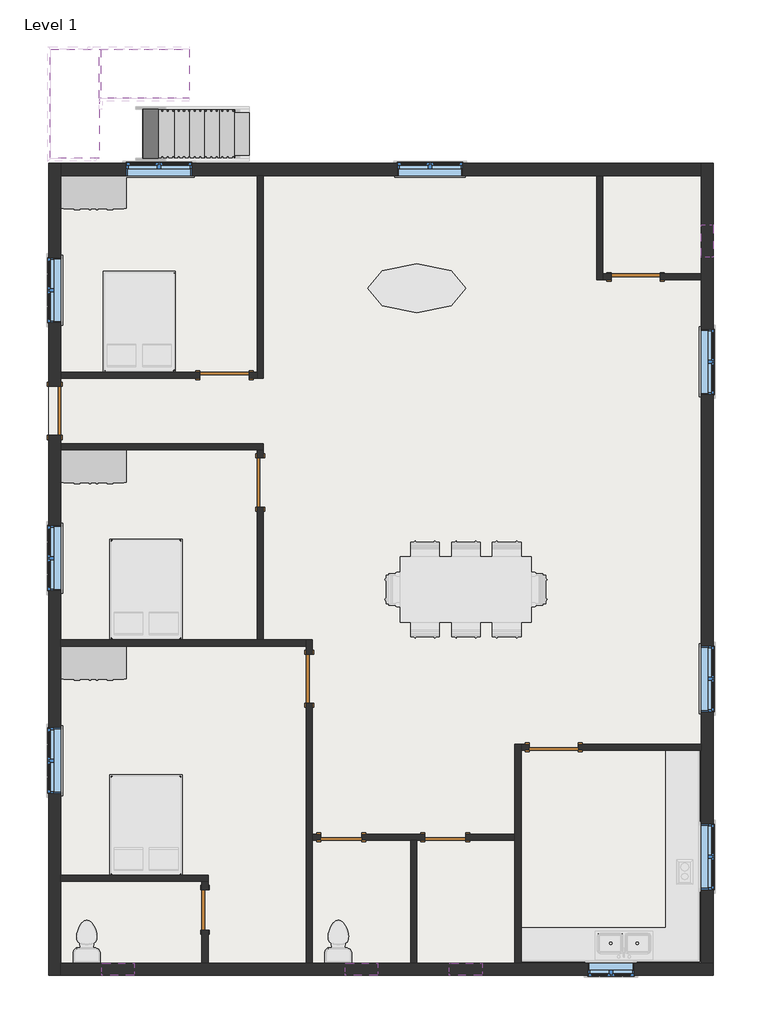
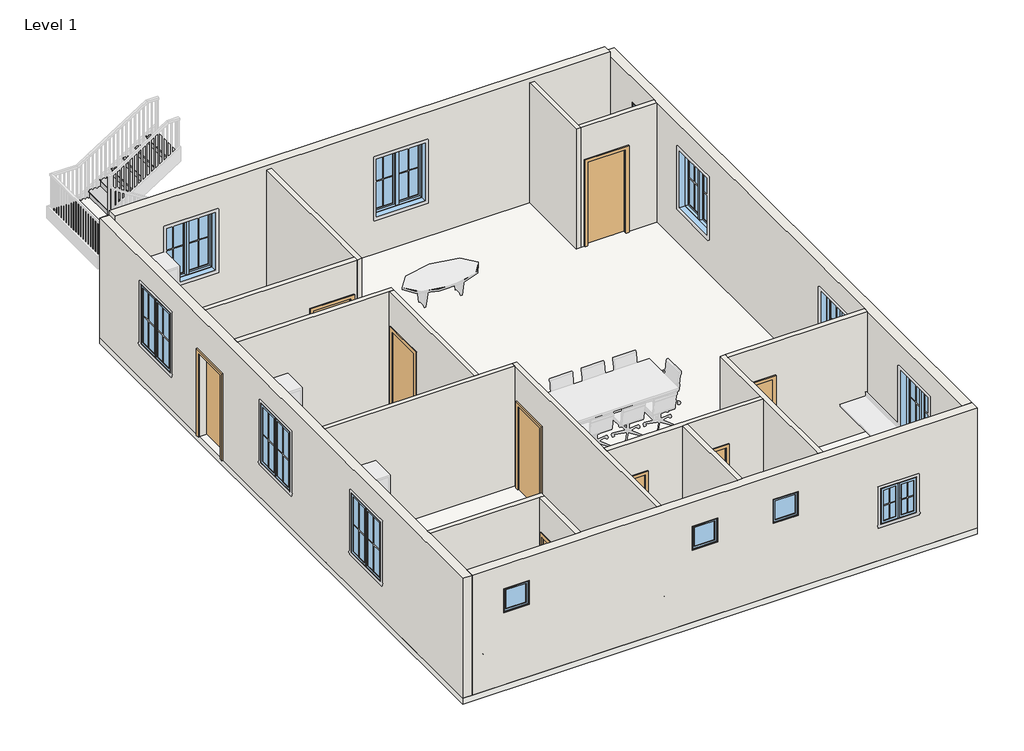
# One storey, part 1 of 3: 18 walls, 13 windows, 9 doors, 2 slabs, 2 stair flights.
"""IFC4 building model written with IfcOpenShell, lengths in millimetres."""

from ifc_helpers import new_model, si_unit, frame, origin, origin_with_axes, place, context, project, spatial, polyline, outline, extrude, faceted_brep, transform, mapped, element, save
from components import door_214872d5, door_a90ba1ad, door_e5f9f3c4, door_305aa2a5, non_monolithic_landing_2ab6d15e, stair_flight_b5a9fedd, stair_flight_7eff537e, window_80340324, window_339605e1, window_8377141f

model = new_model("IFC4")

# Units and contexts
model_context = context("Model", 3, world=origin())
ifc_project = project(units=[si_unit("LENGTHUNIT", "METRE", prefix="MILLI")], contexts=[model_context])

# Site, building, storey
site = spatial("IfcSite", under=ifc_project)
building = spatial("IfcBuilding", under=site)
storey = spatial("IfcBuildingStorey", under=building, Name="Level 1", Elevation=0.0)

# Doors
placement = place(None, origin())
door_shape = door_214872d5(model_context)
element("IfcDoor", 1, ObjectType="Single-Flush : 30\" x 84\"", at=placement, inside=storey, context=model_context, shape_type="MappedRepresentation", body=[
    mapped(door_shape, transform((15054.6713581, 8240.8164065, 0.0), x_axis=(-1.0, 0.0, 0.0), y_axis=(0.0, -1.0, 0.0), z_axis=(0.0, 0.0, 1.0))),
])
element("IfcDoor", 2, ObjectType="Single-Flush : 30\" x 84\"", at=placement, inside=storey, context=model_context, shape_type="MappedRepresentation", body=[
    mapped(door_shape, transform((16997.7713581, 8240.8164065, 0.0), x_axis=(-1.0, 0.0, 0.0), y_axis=(0.0, -1.0, 0.0), z_axis=(0.0, 0.0, 1.0))),
])
element("IfcDoor", 3, ObjectType="Single-Flush : 30\" x 84\"", at=placement, inside=storey, context=model_context, shape_type="MappedRepresentation", body=[
    mapped(door_shape, transform((12521.0213581, 6888.2664065, 0.0), x_axis=(0.0, 1.0, 0.0), y_axis=(-1.0, 0.0, 0.0), z_axis=(0.0, 0.0, 1.0))),
])
door_2_shape = door_a90ba1ad(model_context)
element("IfcDoor", 4, ObjectType="Single-Flush : 36\" x 84\"", at=placement, inside=storey, context=model_context, shape_type="MappedRepresentation", body=[
    mapped(door_2_shape, transform((9720.6713581, 16184.6664065, 0.0), x_axis=(0.0, 1.0, 0.0), y_axis=(-1.0, 0.0, 0.0), z_axis=(0.0, 0.0, 1.0))),
])
door_3_shape = door_e5f9f3c4(model_context)
element("IfcDoor", 5, ObjectType="Single-Flush : 36\" x 84\"", at=placement, inside=storey, context=model_context, shape_type="MappedRepresentation", body=[
    mapped(door_3_shape, transform((12882.9713581, 16851.4164065, 0.0), x_axis=(1.0, 0.0, 0.0), y_axis=(0.0, 1.0, 0.0), z_axis=(0.0, 0.0, 1.0))),
])
element("IfcDoor", 6, ObjectType="Single-Flush : 36\" x 84\"", at=placement, inside=storey, context=model_context, shape_type="MappedRepresentation", body=[
    mapped(door_3_shape, transform((13549.7213581, 14851.1664065, 0.0), x_axis=(0.0, 1.0, 0.0), y_axis=(-1.0, 0.0, 0.0), z_axis=(0.0, 0.0, 1.0))),
])
element("IfcDoor", 7, ObjectType="Single-Flush : 36\" x 84\"", at=placement, inside=storey, context=model_context, shape_type="MappedRepresentation", body=[
    mapped(door_3_shape, transform((14464.1213581, 11193.5664065, 0.0), x_axis=(0.0, 1.0, 0.0), y_axis=(-1.0, 0.0, 0.0), z_axis=(0.0, 0.0, 1.0))),
])
element("IfcDoor", 8, ObjectType="Single-Flush : 36\" x 84\"", at=placement, inside=storey, context=model_context, shape_type="MappedRepresentation", body=[
    mapped(door_3_shape, transform((19017.0713581, 9917.2164065, 0.0), x_axis=(-1.0, 0.0, 0.0), y_axis=(0.0, -1.0, 0.0), z_axis=(0.0, 0.0, 1.0))),
])
door_4_shape = door_305aa2a5(model_context)
element("IfcDoor", 9, ObjectType="Single-Flush : 36\" x 84\"", at=placement, inside=storey, context=model_context, shape_type="MappedRepresentation", body=[
    mapped(door_4_shape, transform((20541.0713581, 18680.2164065, 0.0), x_axis=(-1.0, 0.0, 0.0), y_axis=(0.0, -1.0, 0.0), z_axis=(0.0, 0.0, 1.0))),
])

# Slabs
element("IfcSlab", 10, at=placement, inside=storey, context=model_context, shape_type="SweptSolid", body=[
    extrude(outline(polyline([(21988.8713581, 20794.7664065), (21988.8713581, 5669.0664065), (9606.3713581, 5669.0664065), (9606.3713581, 20794.7664065), (21988.8713581, 20794.7664065)])), frame((0.0, 0.0, -152.4), z_axis=(0.0, 0.0, 1.0), x_axis=(1.0, 0.0, 0.0)), (0.0, 0.0, 1.0), 152.4),
])
non_monolithic_landing_shape = non_monolithic_landing_2ab6d15e(model_context)
element("IfcSlab", 11, ObjectType="Non-Monolithic Landing", at=placement, inside=storey, context=model_context, shape_type="MappedRepresentation", body=[
    mapped(non_monolithic_landing_shape, transform((0.0, 0.0, 0.0), x_axis=(1.0, 0.0, 0.0), y_axis=(0.0, 1.0, 0.0), z_axis=(0.0, 0.0, 1.0))),
])

# Stair flights
stair_flight_shape = stair_flight_b5a9fedd(model_context)
element("IfcStairFlight", 12, ObjectType="2\" Tread 1\" Nosing 1/4\" Riser", at=placement, inside=storey, context=model_context, shape_type="MappedRepresentation", body=[
    mapped(stair_flight_shape, transform((0.0, 0.0, 0.0), x_axis=(1.0, 0.0, 0.0), y_axis=(0.0, 1.0, 0.0), z_axis=(0.0, 0.0, 1.0))),
])
stair_flight_2_shape = stair_flight_7eff537e(model_context)
element("IfcStairFlight", 13, ObjectType="2\" Tread 1\" Nosing 1/4\" Riser", at=placement, inside=storey, context=model_context, shape_type="MappedRepresentation", body=[
    mapped(stair_flight_2_shape, transform((0.0, 0.0, 0.0), x_axis=(1.0, 0.0, 0.0), y_axis=(0.0, 1.0, 0.0), z_axis=(0.0, 0.0, 1.0))),
])

# Walls
element("IfcWall", 14, at=placement, inside=storey, context=model_context, shape_type="Brep", body=[
    faceted_brep([(9606.3713581, 20794.7664065, 0.0), (9606.3713581, 16641.8664065, 0.0), (9606.3713581, 16641.8664065, 2133.6), (9606.3713581, 15727.4664065, 2133.6), (9606.3713581, 15727.4664065, 0.0), (9606.3713581, 5669.0664065, 0.0), (9606.3713581, 5669.0664065, 3048.0), (9606.3713581, 20788.4164065, 3048.0), (9606.3713581, 20794.7664065, 3048.0), (9606.3713581, 19042.1664065, 2438.4), (9606.3713581, 17822.9664065, 2438.4), (9606.3713581, 17822.9664065, 914.4), (9606.3713581, 19042.1664065, 914.4), (9606.3713581, 14051.0664065, 2438.4), (9606.3713581, 12831.8664065, 2438.4), (9606.3713581, 12831.8664065, 914.4), (9606.3713581, 14051.0664065, 914.4), (9606.3713581, 10279.1664065, 2438.4), (9606.3713581, 9059.9664065, 2438.4), (9606.3713581, 9059.9664065, 914.4), (9606.3713581, 10279.1664065, 914.4), (9834.9713581, 16641.8664065, 2133.6), (9834.9713581, 16641.8664065, 0.0), (9834.9713581, 16794.2664065, 0.0), (9834.9713581, 16908.5664065, 0.0), (9834.9713581, 20566.1664065, 0.0), (9834.9713581, 20794.7664065, 0.0), (9834.9713581, 20794.7664065, 3048.0), (9834.9713581, 20788.4164065, 3048.0), (9834.9713581, 16908.5664065, 3048.0), (9834.9713581, 16794.2664065, 3048.0), (9834.9713581, 15575.0664065, 3048.0), (9834.9713581, 15460.7664065, 3048.0), (9834.9713581, 11917.4664065, 3048.0), (9834.9713581, 11803.1664065, 3048.0), (9834.9713581, 7535.9664065, 3048.0), (9834.9713581, 7421.6664065, 3048.0), (9834.9713581, 5897.6664065, 3048.0), (9834.9713581, 5669.0664065, 3048.0), (9834.9713581, 5669.0664065, 0.0), (9834.9713581, 5897.6664065, 0.0), (9834.9713581, 7421.6664065, 0.0), (9834.9713581, 7535.9664065, 0.0), (9834.9713581, 11803.1664065, 0.0), (9834.9713581, 11917.4664065, 0.0), (9834.9713581, 15460.7664065, 0.0), (9834.9713581, 15575.0664065, 0.0), (9834.9713581, 15727.4664065, 0.0), (9834.9713581, 15727.4664065, 2133.6), (9834.9713581, 19042.1664065, 2438.4), (9834.9713581, 19042.1664065, 914.4), (9834.9713581, 17822.9664065, 914.4), (9834.9713581, 17822.9664065, 2438.4), (9834.9713581, 14051.0664065, 2438.4), (9834.9713581, 14051.0664065, 914.4), (9834.9713581, 12831.8664065, 914.4), (9834.9713581, 12831.8664065, 2438.4), (9834.9713581, 10279.1664065, 2438.4), (9834.9713581, 10279.1664065, 914.4), (9834.9713581, 9059.9664065, 914.4), (9834.9713581, 9059.9664065, 2438.4)], [[[0, 1, 2, 3, 4, 5, 6, 7, 8], [9, 10, 11, 12], [13, 14, 15, 16], [17, 18, 19, 20]], [[21, 22, 23, 24, 25, 26, 27, 28, 29, 30, 31, 32, 33, 34, 35, 36, 37, 38, 39, 40, 41, 42, 43, 44, 45, 46, 47, 48], [49, 50, 51, 52], [53, 54, 55, 56], [57, 58, 59, 60]], [[26, 25, 24, 23, 22, 1, 0]], [[47, 46, 45, 44, 43, 42, 41, 40, 39, 5, 4]], [[0, 8, 27, 26]], [[6, 5, 39, 38]], [[2, 1, 22, 21]], [[3, 2, 21, 48]], [[4, 3, 48, 47]], [[50, 49, 9, 12]], [[51, 50, 12, 11]], [[52, 51, 11, 10]], [[49, 52, 10, 9]], [[54, 53, 13, 16]], [[55, 54, 16, 15]], [[56, 55, 15, 14]], [[53, 56, 14, 13]], [[58, 57, 17, 20]], [[59, 58, 20, 19]], [[60, 59, 19, 18]], [[57, 60, 18, 17]], [[8, 7, 28, 27]], [[7, 6, 38, 37, 36, 35, 34, 33, 32, 31, 30, 29, 28]]]),
])
element("IfcWall", 15, at=placement, inside=storey, context=model_context, shape_type="Brep", body=[
    faceted_brep([(9834.9713581, 20566.1664065, 0.0), (13492.5713581, 20566.1664065, 0.0), (13606.8713581, 20566.1664065, 0.0), (19817.1713581, 20566.1664065, 0.0), (19931.4713581, 20566.1664065, 0.0), (21760.2713581, 20566.1664065, 0.0), (21760.2713581, 20566.1664065, 3155.7444843), (9834.9713581, 20566.1664065, 3155.7444843), (12273.3713581, 20566.1664065, 2438.4), (12273.3713581, 20566.1664065, 914.4), (11054.1713581, 20566.1664065, 914.4), (11054.1713581, 20566.1664065, 2438.4), (17321.6213581, 20566.1664065, 2438.4), (17321.6213581, 20566.1664065, 914.4), (16102.4213581, 20566.1664065, 914.4), (16102.4213581, 20566.1664065, 2438.4), (9834.9713581, 20794.7664065, 0.0), (9834.9713581, 20794.7664065, 3048.0), (9834.9713581, 20794.7664065, 3155.7444843), (21760.2713581, 20794.7664065, 3155.7444843), (21760.2713581, 20794.7664065, 3048.0), (21760.2713581, 20794.7664065, 0.0), (12273.3713581, 20794.7664065, 2438.4), (11054.1713581, 20794.7664065, 2438.4), (11054.1713581, 20794.7664065, 914.4), (12273.3713581, 20794.7664065, 914.4), (17321.6213581, 20794.7664065, 2438.4), (16102.4213581, 20794.7664065, 2438.4), (16102.4213581, 20794.7664065, 914.4), (17321.6213581, 20794.7664065, 914.4)], [[[0, 1, 2, 3, 4, 5, 6, 7], [8, 9, 10, 11], [12, 13, 14, 15]], [[16, 17, 18, 19, 20, 21], [22, 23, 24, 25], [26, 27, 28, 29]], [[5, 4, 3, 2, 1, 0, 16, 21]], [[7, 6, 19, 18]], [[0, 7, 18, 17, 16]], [[6, 5, 21, 20, 19]], [[9, 8, 22, 25]], [[10, 9, 25, 24]], [[11, 10, 24, 23]], [[8, 11, 23, 22]], [[13, 12, 26, 29]], [[14, 13, 29, 28]], [[15, 14, 28, 27]], [[12, 15, 27, 26]]]),
])
element("IfcWall", 16, at=placement, inside=storey, context=model_context, shape_type="Brep", body=[
    faceted_brep([(13492.5713581, 20566.1664065, 0.0), (13492.5713581, 16908.5664065, 0.0), (13492.5713581, 16794.2664065, 0.0), (13492.5713581, 16794.2664065, 3048.0), (13492.5713581, 16908.5664065, 3048.0), (13492.5713581, 20566.1664065, 3048.0), (13606.8713581, 20566.1664065, 0.0), (13606.8713581, 20566.1664065, 3048.0), (13606.8713581, 16794.2664065, 3048.0), (13606.8713581, 16794.2664065, 0.0)], [[[0, 1, 2, 3, 4, 5]], [[6, 7, 8, 9]], [[2, 1, 0, 6, 9]], [[3, 2, 9, 8]], [[0, 5, 7, 6]], [[5, 4, 3, 8, 7]]]),
])
element("IfcWall", 17, at=placement, inside=storey, context=model_context, shape_type="SweptSolid", body=[
    extrude(outline(polyline([(2133.6, 13340.1713581), (0.0, 13340.1713581), (0.0, 13492.5713581), (3048.0, 13492.5713581), (3048.0, 9834.9713581), (0.0, 9834.9713581), (0.0, 12425.7713581), (2133.6, 12425.7713581), (2133.6, 13340.1713581)])), frame((0.0, 16794.2664065, 0.0), z_axis=(0.0, 1.0, 0.0), x_axis=(0.0, 0.0, 1.0)), (0.0, 0.0, 1.0), 114.3),
])
element("IfcWall", 18, at=placement, inside=storey, context=model_context, shape_type="Brep", body=[
    faceted_brep([(9834.9713581, 15460.7664065, 0.0), (13492.5713581, 15460.7664065, 0.0), (13606.8713581, 15460.7664065, 0.0), (13606.8713581, 15460.7664065, 3048.0), (13492.5713581, 15460.7664065, 3048.0), (9834.9713581, 15460.7664065, 3048.0), (9834.9713581, 15575.0664065, 0.0), (9834.9713581, 15575.0664065, 3048.0), (13606.8713581, 15575.0664065, 3048.0), (13606.8713581, 15575.0664065, 0.0)], [[[0, 1, 2, 3, 4, 5]], [[6, 7, 8, 9]], [[2, 1, 0, 6, 9]], [[0, 5, 7, 6]], [[3, 2, 9, 8]], [[5, 4, 3, 8, 7]]]),
])
element("IfcWall", 19, at=placement, inside=storey, context=model_context, shape_type="Brep", body=[
    faceted_brep([(9834.9713581, 11803.1664065, 0.0), (14406.9713581, 11803.1664065, 0.0), (14406.9713581, 11803.1664065, 3048.0), (9834.9713581, 11803.1664065, 3048.0), (9834.9713581, 11917.4664065, 0.0), (9834.9713581, 11917.4664065, 3048.0), (13492.5713581, 11917.4664065, 3048.0), (13606.8713581, 11917.4664065, 3048.0), (14406.9713581, 11917.4664065, 3048.0), (14406.9713581, 11917.4664065, 0.0), (13606.8713581, 11917.4664065, 0.0), (13492.5713581, 11917.4664065, 0.0)], [[[0, 1, 2, 3]], [[4, 5, 6, 7, 8, 9, 10, 11]], [[1, 0, 4, 11, 10, 9]], [[0, 3, 5, 4]], [[2, 1, 9, 8]], [[3, 2, 8, 7, 6, 5]]]),
])
element("IfcWall", 20, at=placement, inside=storey, context=model_context, shape_type="SweptSolid", body=[
    extrude(outline(polyline([(15460.7664065, 0.0), (15308.3664065, 0.0), (15308.3664065, 2133.6), (14393.9664065, 2133.6), (14393.9664065, 0.0), (11917.4664065, 0.0), (11917.4664065, 3048.0), (15460.7664065, 3048.0), (15460.7664065, 0.0)])), frame((13492.5713581, 0.0, 0.0), z_axis=(1.0, 0.0, 0.0), x_axis=(0.0, 1.0, 0.0)), (0.0, 0.0, 1.0), 114.3),
])
element("IfcWall", 21, at=placement, inside=storey, context=model_context, shape_type="Brep", body=[
    faceted_brep([(9834.9713581, 7421.6664065, 0.0), (12463.8713581, 7421.6664065, 0.0), (12578.1713581, 7421.6664065, 0.0), (12578.1713581, 7421.6664065, 3048.0), (12463.8713581, 7421.6664065, 3048.0), (9834.9713581, 7421.6664065, 3048.0), (9834.9713581, 7535.9664065, 0.0), (9834.9713581, 7535.9664065, 3048.0), (12578.1713581, 7535.9664065, 3048.0), (12578.1713581, 7535.9664065, 0.0)], [[[0, 1, 2, 3, 4, 5]], [[6, 7, 8, 9]], [[2, 1, 0, 6, 9]], [[0, 5, 7, 6]], [[5, 4, 3, 8, 7]], [[3, 2, 9, 8]]]),
])
element("IfcWall", 22, at=placement, inside=storey, context=model_context, shape_type="Brep", body=[
    faceted_brep([(14521.2713581, 11650.7664065, 2133.6), (14521.2713581, 11650.7664065, 0.0), (14521.2713581, 11917.4664065, 0.0), (14521.2713581, 11917.4664065, 3048.0), (14521.2713581, 8297.9664065, 3048.0), (14521.2713581, 8183.6664065, 3048.0), (14521.2713581, 5897.6664065, 3048.0), (14521.2713581, 5897.6664065, 0.0), (14521.2713581, 8183.6664065, 0.0), (14521.2713581, 8297.9664065, 0.0), (14521.2713581, 10736.3664065, 0.0), (14521.2713581, 10736.3664065, 2133.6), (14406.9713581, 11917.4664065, 0.0), (14406.9713581, 11803.1664065, 0.0), (14406.9713581, 11650.7664065, 0.0), (14406.9713581, 11650.7664065, 2133.6), (14406.9713581, 10736.3664065, 2133.6), (14406.9713581, 10736.3664065, 0.0), (14406.9713581, 5897.6664065, 0.0), (14406.9713581, 5897.6664065, 3048.0), (14406.9713581, 11803.1664065, 3048.0), (14406.9713581, 11917.4664065, 3048.0)], [[[0, 1, 2, 3, 4, 5, 6, 7, 8, 9, 10, 11]], [[12, 13, 14, 15, 16, 17, 18, 19, 20, 21]], [[2, 1, 14, 13, 12]], [[10, 9, 8, 7, 18, 17]], [[3, 2, 12, 21]], [[7, 6, 19, 18]], [[15, 14, 1, 0]], [[16, 15, 0, 11]], [[17, 16, 11, 10]], [[6, 5, 4, 3, 21, 20, 19]]]),
])
element("IfcWall", 23, at=placement, inside=storey, context=model_context, shape_type="Brep", body=[
    faceted_brep([(9834.9713581, 5669.0664065, 0.0), (21988.8713581, 5669.0664065, 0.0), (21988.8713581, 5669.0664065, 3048.0), (9834.9713581, 5669.0664065, 3048.0), (10596.9713581, 5669.0664065, 2438.4), (11206.5713581, 5669.0664065, 2438.4), (11206.5713581, 5669.0664065, 1828.8), (10596.9713581, 5669.0664065, 1828.8), (15130.8713581, 5669.0664065, 2438.4), (15740.4713581, 5669.0664065, 2438.4), (15740.4713581, 5669.0664065, 1828.8), (15130.8713581, 5669.0664065, 1828.8), (17073.9713581, 5669.0664065, 2438.4), (17683.5713581, 5669.0664065, 2438.4), (17683.5713581, 5669.0664065, 1828.8), (17073.9713581, 5669.0664065, 1828.8), (19652.0713581, 5669.0664065, 1828.8), (20515.6713581, 5669.0664065, 1828.8), (20515.6713581, 5669.0664065, 914.4), (19652.0713581, 5669.0664065, 914.4), (9834.9713581, 5897.6664065, 0.0), (9834.9713581, 5897.6664065, 3048.0), (12463.8713581, 5897.6664065, 3048.0), (12578.1713581, 5897.6664065, 3048.0), (14406.9713581, 5897.6664065, 3048.0), (14521.2713581, 5897.6664065, 3048.0), (16350.0713581, 5897.6664065, 3048.0), (16464.3713581, 5897.6664065, 3048.0), (18293.1713581, 5897.6664065, 3048.0), (18407.4713581, 5897.6664065, 3048.0), (21760.2713581, 5897.6664065, 3048.0), (21988.8713581, 5897.6664065, 3048.0), (21988.8713581, 5897.6664065, 0.0), (21760.2713581, 5897.6664065, 0.0), (18407.4713581, 5897.6664065, 0.0), (18293.1713581, 5897.6664065, 0.0), (16464.3713581, 5897.6664065, 0.0), (16350.0713581, 5897.6664065, 0.0), (14521.2713581, 5897.6664065, 0.0), (14406.9713581, 5897.6664065, 0.0), (12578.1713581, 5897.6664065, 0.0), (12463.8713581, 5897.6664065, 0.0), (10596.9713581, 5897.6664065, 2438.4), (10596.9713581, 5897.6664065, 1828.8), (11206.5713581, 5897.6664065, 1828.8), (11206.5713581, 5897.6664065, 2438.4), (15130.8713581, 5897.6664065, 2438.4), (15130.8713581, 5897.6664065, 1828.8), (15740.4713581, 5897.6664065, 1828.8), (15740.4713581, 5897.6664065, 2438.4), (17073.9713581, 5897.6664065, 2438.4), (17073.9713581, 5897.6664065, 1828.8), (17683.5713581, 5897.6664065, 1828.8), (17683.5713581, 5897.6664065, 2438.4), (19652.0713581, 5897.6664065, 1828.8), (19652.0713581, 5897.6664065, 914.4), (20515.6713581, 5897.6664065, 914.4), (20515.6713581, 5897.6664065, 1828.8)], [[[0, 1, 2, 3], [4, 5, 6, 7], [8, 9, 10, 11], [12, 13, 14, 15], [16, 17, 18, 19]], [[20, 21, 22, 23, 24, 25, 26, 27, 28, 29, 30, 31, 32, 33, 34, 35, 36, 37, 38, 39, 40, 41], [42, 43, 44, 45], [46, 47, 48, 49], [50, 51, 52, 53], [54, 55, 56, 57]], [[1, 0, 20, 41, 40, 39, 38, 37, 36, 35, 34, 33, 32]], [[0, 3, 21, 20]], [[2, 1, 32, 31]], [[43, 42, 4, 7]], [[44, 43, 7, 6]], [[45, 44, 6, 5]], [[42, 45, 5, 4]], [[47, 46, 8, 11]], [[48, 47, 11, 10]], [[49, 48, 10, 9]], [[46, 49, 9, 8]], [[51, 50, 12, 15]], [[52, 51, 15, 14]], [[53, 52, 14, 13]], [[50, 53, 13, 12]], [[55, 54, 16, 19]], [[56, 55, 19, 18]], [[57, 56, 18, 17]], [[54, 57, 17, 16]], [[3, 2, 31, 30, 29, 28, 27, 26, 25, 24, 23, 22, 21]]]),
])
element("IfcWall", 24, at=placement, inside=storey, context=model_context, shape_type="SweptSolid", body=[
    extrude(outline(polyline([(16464.3713581, 8183.6664065), (16464.3713581, 5897.6664065), (16350.0713581, 5897.6664065), (16350.0713581, 8183.6664065), (16464.3713581, 8183.6664065)])), origin_with_axes(), (0.0, 0.0, 1.0), 3048.0),
])
element("IfcWall", 25, at=placement, inside=storey, context=model_context, shape_type="Brep", body=[
    faceted_brep([(16616.7713581, 8297.9664065, 2133.6), (16616.7713581, 8297.9664065, 0.0), (15435.6713581, 8297.9664065, 0.0), (15435.6713581, 8297.9664065, 2133.6), (14673.6713581, 8297.9664065, 2133.6), (14673.6713581, 8297.9664065, 0.0), (14521.2713581, 8297.9664065, 0.0), (14521.2713581, 8297.9664065, 3048.0), (18293.1713581, 8297.9664065, 3048.0), (18293.1713581, 8297.9664065, 0.0), (17378.7713581, 8297.9664065, 0.0), (17378.7713581, 8297.9664065, 2133.6), (15435.6713581, 8183.6664065, 0.0), (16350.0713581, 8183.6664065, 0.0), (16464.3713581, 8183.6664065, 0.0), (16616.7713581, 8183.6664065, 0.0), (16616.7713581, 8183.6664065, 2133.6), (17378.7713581, 8183.6664065, 2133.6), (17378.7713581, 8183.6664065, 0.0), (18293.1713581, 8183.6664065, 0.0), (18293.1713581, 8183.6664065, 3048.0), (16464.3713581, 8183.6664065, 3048.0), (16350.0713581, 8183.6664065, 3048.0), (14521.2713581, 8183.6664065, 3048.0), (14521.2713581, 8183.6664065, 0.0), (14673.6713581, 8183.6664065, 0.0), (14673.6713581, 8183.6664065, 2133.6), (15435.6713581, 8183.6664065, 2133.6)], [[[0, 1, 2, 3, 4, 5, 6, 7, 8, 9, 10, 11]], [[12, 13, 14, 15, 16, 17, 18, 19, 20, 21, 22, 23, 24, 25, 26, 27]], [[6, 5, 25, 24]], [[10, 9, 19, 18]], [[2, 1, 15, 14, 13, 12]], [[7, 6, 24, 23]], [[9, 8, 20, 19]], [[26, 25, 5, 4]], [[27, 26, 4, 3]], [[12, 27, 3, 2]], [[16, 15, 1, 0]], [[17, 16, 0, 11]], [[18, 17, 11, 10]], [[8, 7, 23, 22, 21, 20]]]),
])
element("IfcWall", 26, at=placement, inside=storey, context=model_context, shape_type="Brep", body=[
    faceted_brep([(18293.1713581, 9974.3664065, 0.0), (18293.1713581, 8297.9664065, 0.0), (18293.1713581, 8183.6664065, 0.0), (18293.1713581, 5897.6664065, 0.0), (18293.1713581, 5897.6664065, 3048.0), (18293.1713581, 8183.6664065, 3048.0), (18293.1713581, 8297.9664065, 3048.0), (18293.1713581, 9974.3664065, 3048.0), (18407.4713581, 9974.3664065, 0.0), (18407.4713581, 9974.3664065, 3048.0), (18407.4713581, 9860.0664065, 3048.0), (18407.4713581, 5897.6664065, 3048.0), (18407.4713581, 5897.6664065, 0.0), (18407.4713581, 9860.0664065, 0.0)], [[[0, 1, 2, 3, 4, 5, 6, 7]], [[8, 9, 10, 11, 12, 13]], [[3, 2, 1, 0, 8, 13, 12]], [[4, 3, 12, 11]], [[0, 7, 9, 8]], [[7, 6, 5, 4, 11, 10, 9]]]),
])
element("IfcWall", 27, at=placement, inside=storey, context=model_context, shape_type="Brep", body=[
    faceted_brep([(21988.8713581, 5897.6664065, 0.0), (21988.8713581, 20794.7664065, 0.0), (21988.8713581, 20794.7664065, 3048.0), (21988.8713581, 5897.6664065, 3048.0), (21988.8713581, 10583.9664065, 2438.4), (21988.8713581, 11803.1664065, 2438.4), (21988.8713581, 11803.1664065, 914.4), (21988.8713581, 10583.9664065, 914.4), (21988.8713581, 16489.4664065, 2438.4), (21988.8713581, 17708.6664065, 2438.4), (21988.8713581, 17708.6664065, 914.4), (21988.8713581, 16489.4664065, 914.4), (21988.8713581, 19042.1664065, 2438.4), (21988.8713581, 19651.7664065, 2438.4), (21988.8713581, 19651.7664065, 1828.8), (21988.8713581, 19042.1664065, 1828.8), (21988.8713581, 7269.2664065, 2438.4), (21988.8713581, 8488.4664065, 2438.4), (21988.8713581, 8488.4664065, 914.4), (21988.8713581, 7269.2664065, 914.4), (21760.2713581, 5897.6664065, 0.0), (21760.2713581, 5897.6664065, 3048.0), (21760.2713581, 9860.0664065, 3048.0), (21760.2713581, 9974.3664065, 3048.0), (21760.2713581, 18623.0664065, 3048.0), (21760.2713581, 18737.3664065, 3048.0), (21760.2713581, 20794.7664065, 3048.0), (21760.2713581, 20794.7664065, 0.0), (21760.2713581, 20566.1664065, 0.0), (21760.2713581, 18737.3664065, 0.0), (21760.2713581, 18623.0664065, 0.0), (21760.2713581, 9974.3664065, 0.0), (21760.2713581, 9860.0664065, 0.0), (21760.2713581, 10583.9664065, 2438.4), (21760.2713581, 10583.9664065, 914.4), (21760.2713581, 11803.1664065, 914.4), (21760.2713581, 11803.1664065, 2438.4), (21760.2713581, 16489.4664065, 2438.4), (21760.2713581, 16489.4664065, 914.4), (21760.2713581, 17708.6664065, 914.4), (21760.2713581, 17708.6664065, 2438.4), (21760.2713581, 19042.1664065, 2438.4), (21760.2713581, 19042.1664065, 1828.8), (21760.2713581, 19651.7664065, 1828.8), (21760.2713581, 19651.7664065, 2438.4), (21760.2713581, 7269.2664065, 2438.4), (21760.2713581, 7269.2664065, 914.4), (21760.2713581, 8488.4664065, 914.4), (21760.2713581, 8488.4664065, 2438.4)], [[[0, 1, 2, 3], [4, 5, 6, 7], [8, 9, 10, 11], [12, 13, 14, 15], [16, 17, 18, 19]], [[20, 21, 22, 23, 24, 25, 26, 27, 28, 29, 30, 31, 32], [33, 34, 35, 36], [37, 38, 39, 40], [41, 42, 43, 44], [45, 46, 47, 48]], [[1, 0, 20, 32, 31, 30, 29, 28, 27]], [[0, 3, 21, 20]], [[2, 1, 27, 26]], [[34, 33, 4, 7]], [[35, 34, 7, 6]], [[36, 35, 6, 5]], [[33, 36, 5, 4]], [[38, 37, 8, 11]], [[39, 38, 11, 10]], [[40, 39, 10, 9]], [[37, 40, 9, 8]], [[42, 41, 12, 15]], [[43, 42, 15, 14]], [[44, 43, 14, 13]], [[41, 44, 13, 12]], [[46, 45, 16, 19]], [[47, 46, 19, 18]], [[48, 47, 18, 17]], [[45, 48, 17, 16]], [[3, 2, 26, 25, 24, 23, 22, 21]]]),
])
element("IfcWall", 28, at=placement, inside=storey, context=model_context, shape_type="SweptSolid", body=[
    extrude(outline(polyline([(0.0, 18407.4713581), (0.0, 18559.8713581), (2133.6, 18559.8713581), (2133.6, 19474.2713581), (0.0, 19474.2713581), (0.0, 21760.2713581), (3048.0, 21760.2713581), (3048.0, 18407.4713581), (0.0, 18407.4713581)])), frame((0.0, 9860.0664065, 0.0), z_axis=(0.0, 1.0, 0.0), x_axis=(0.0, 0.0, 1.0)), (0.0, 0.0, 1.0), 114.3),
])
element("IfcWall", 29, at=placement, inside=storey, context=model_context, shape_type="Brep", body=[
    faceted_brep([(19817.1713581, 20566.1664065, 0.0), (19817.1713581, 18623.0664065, 0.0), (19817.1713581, 18623.0664065, 3048.0), (19817.1713581, 20566.1664065, 3048.0), (19931.4713581, 20566.1664065, 0.0), (19931.4713581, 20566.1664065, 3048.0), (19931.4713581, 18737.3664065, 3048.0), (19931.4713581, 18623.0664065, 3048.0), (19931.4713581, 18623.0664065, 0.0), (19931.4713581, 18737.3664065, 0.0)], [[[0, 1, 2, 3]], [[4, 5, 6, 7, 8, 9]], [[1, 0, 4, 9, 8]], [[0, 3, 5, 4]], [[2, 1, 8, 7]], [[3, 2, 7, 6, 5]]]),
])
element("IfcWall", 30, at=placement, inside=storey, context=model_context, shape_type="SweptSolid", body=[
    extrude(outline(polyline([(0.0, 19931.4713581), (0.0, 20083.8713581), (2133.6, 20083.8713581), (2133.6, 20998.2713581), (0.0, 20998.2713581), (0.0, 21760.2713581), (3048.0, 21760.2713581), (3048.0, 19931.4713581), (0.0, 19931.4713581)])), frame((0.0, 18623.0664065, 0.0), z_axis=(0.0, 1.0, 0.0), x_axis=(0.0, 0.0, 1.0)), (0.0, 0.0, 1.0), 114.3),
])
element("IfcWall", 31, at=placement, inside=storey, context=model_context, shape_type="SweptSolid", body=[
    extrude(outline(polyline([(5897.6664065, 0.0), (5897.6664065, 3048.0), (7421.6664065, 3048.0), (7421.6664065, 0.0), (7269.2664065, 0.0), (7269.2664065, 2133.6), (6507.2664065, 2133.6), (6507.2664065, 0.0), (5897.6664065, 0.0)])), frame((12463.8713581, 0.0, 0.0), z_axis=(1.0, 0.0, 0.0), x_axis=(0.0, 1.0, 0.0)), (0.0, 0.0, 1.0), 114.3),
])

# Windows
window_shape = window_80340324(model_context)
element("IfcWindow", 32, ObjectType="Fixed : 24\" x 24\"", at=placement, inside=storey, context=model_context, shape_type="MappedRepresentation", body=[
    mapped(window_shape, transform((10863.6713581, 5783.3664065, 914.4), x_axis=(-1.0, 0.0, 0.0), y_axis=(0.0, -1.0, 0.0), z_axis=(0.0, 0.0, 1.0))),
])
element("IfcWindow", 33, ObjectType="Fixed : 24\" x 24\"", at=placement, inside=storey, context=model_context, shape_type="MappedRepresentation", body=[
    mapped(window_shape, transform((15397.5713581, 5783.3664065, 914.4), x_axis=(-1.0, 0.0, 0.0), y_axis=(0.0, -1.0, 0.0), z_axis=(0.0, 0.0, 1.0))),
])
element("IfcWindow", 34, ObjectType="Fixed : 24\" x 24\"", at=placement, inside=storey, context=model_context, shape_type="MappedRepresentation", body=[
    mapped(window_shape, transform((17340.6713581, 5783.3664065, 914.4), x_axis=(-1.0, 0.0, 0.0), y_axis=(0.0, -1.0, 0.0), z_axis=(0.0, 0.0, 1.0))),
])
element("IfcWindow", 35, ObjectType="Fixed : 24\" x 24\"", at=placement, inside=storey, context=model_context, shape_type="MappedRepresentation", body=[
    mapped(window_shape, transform((21874.5713581, 19308.8664065, 914.4), x_axis=(0.0, -1.0, 0.0), y_axis=(1.0, 0.0, 0.0), z_axis=(0.0, 0.0, 1.0))),
])
window_2_shape = window_339605e1(model_context)
element("IfcWindow", 36, ObjectType="Window-Casement-Double : 34\" x 36\"", at=placement, inside=storey, context=model_context, shape_type="MappedRepresentation", body=[
    mapped(window_2_shape, transform((20083.8713581, 5783.3664065, 0.0), x_axis=(-1.0, 0.0, 0.0), y_axis=(0.0, -1.0, 0.0), z_axis=(0.0, 0.0, 1.0))),
])
window_3_shape = window_8377141f(model_context)
element("IfcWindow", 37, ObjectType="Window-Casement-Double : 48\" x 60\"", at=placement, inside=storey, context=model_context, shape_type="MappedRepresentation", body=[
    mapped(window_3_shape, transform((9720.6713581, 18432.5664065, 0.0), x_axis=(0.0, 1.0, 0.0), y_axis=(-1.0, 0.0, 0.0), z_axis=(0.0, 0.0, 1.0))),
])
element("IfcWindow", 38, ObjectType="Window-Casement-Double : 48\" x 60\"", at=placement, inside=storey, context=model_context, shape_type="MappedRepresentation", body=[
    mapped(window_3_shape, transform((11663.7713581, 20680.4664065, 0.0), x_axis=(1.0, 0.0, 0.0), y_axis=(0.0, 1.0, 0.0), z_axis=(0.0, 0.0, 1.0))),
])
element("IfcWindow", 39, ObjectType="Window-Casement-Double : 48\" x 60\"", at=placement, inside=storey, context=model_context, shape_type="MappedRepresentation", body=[
    mapped(window_3_shape, transform((9720.6713581, 13441.4664065, 0.0), x_axis=(0.0, 1.0, 0.0), y_axis=(-1.0, 0.0, 0.0), z_axis=(0.0, 0.0, 1.0))),
])
element("IfcWindow", 40, ObjectType="Window-Casement-Double : 48\" x 60\"", at=placement, inside=storey, context=model_context, shape_type="MappedRepresentation", body=[
    mapped(window_3_shape, transform((9720.6713581, 9669.5664065, 0.0), x_axis=(0.0, 1.0, 0.0), y_axis=(-1.0, 0.0, 0.0), z_axis=(0.0, 0.0, 1.0))),
])
element("IfcWindow", 41, ObjectType="Window-Casement-Double : 48\" x 60\"", at=placement, inside=storey, context=model_context, shape_type="MappedRepresentation", body=[
    mapped(window_3_shape, transform((21874.5713581, 11193.5664065, 0.0), x_axis=(0.0, -1.0, 0.0), y_axis=(1.0, 0.0, 0.0), z_axis=(0.0, 0.0, 1.0))),
])
element("IfcWindow", 42, ObjectType="Window-Casement-Double : 48\" x 60\"", at=placement, inside=storey, context=model_context, shape_type="MappedRepresentation", body=[
    mapped(window_3_shape, transform((21874.5713581, 17099.0664065, 0.0), x_axis=(0.0, -1.0, 0.0), y_axis=(1.0, 0.0, 0.0), z_axis=(0.0, 0.0, 1.0))),
])
element("IfcWindow", 43, ObjectType="Window-Casement-Double : 48\" x 60\"", at=placement, inside=storey, context=model_context, shape_type="MappedRepresentation", body=[
    mapped(window_3_shape, transform((16712.0213581, 20680.4664065, 0.0), x_axis=(1.0, 0.0, 0.0), y_axis=(0.0, 1.0, 0.0), z_axis=(0.0, 0.0, 1.0))),
])
element("IfcWindow", 44, ObjectType="Window-Casement-Double : 48\" x 60\"", at=placement, inside=storey, context=model_context, shape_type="MappedRepresentation", body=[
    mapped(window_3_shape, transform((21874.5713581, 7878.8664065, 0.0), x_axis=(0.0, -1.0, 0.0), y_axis=(1.0, 0.0, 0.0), z_axis=(0.0, 0.0, 1.0))),
])

save(model, "model.ifc")

# Revit data of these elements
# Type "Single-Flush : 30\" x 84\""
#   Type Mark = "4"
#   Construction Type Id = "MDOOR"
#   Assembly Code = "C1020"
#   Analytic Construction = "Metal"
#   Thickness = 0' - 2"
#   Heat Transfer Coefficient (U) = 0.651978 BTU/(h·ft²·°F)
#   Height = 7' - 0"
#   Trim Projection Ext = 0' - 1"
#   Trim Projection Int = 0' - 1"
#   Trim Width = 0' - 3"
#   Width = 2' - 6"
#   Define Thermal Properties by = 1
#   Define Thermal Properties by = 1
#   Door Material = Door - Panel
#   Frame Material = Door - Frame
#   Visual Light Transmittance = 0
#   Solar Heat Gain Coefficient = 0
#   Function = (empty or 0)
#   Wall Closure = (empty or 0)
# Type "Single-Flush : 36\" x 84\""
#   Type Mark = "1"
#   Construction Type Id = "MDOOR"
#   Assembly Code = "C1020"
#   Analytic Construction = "Metal"
#   Thickness = 0' - 2"
#   Heat Transfer Coefficient (U) = 0.651978 BTU/(h·ft²·°F)
#   Height = 7' - 0"
#   Trim Projection Ext = 0' - 1"
#   Trim Projection Int = 0' - 1"
#   Trim Width = 0' - 3"
#   Width = 3' - 0"
#   Define Thermal Properties by = 1
#   Define Thermal Properties by = 1
#   Door Material = Door - Panel
#   Frame Material = Door - Frame
#   Visual Light Transmittance = 0
#   Solar Heat Gain Coefficient = 0
#   Function = (empty or 0)
#   Wall Closure = (empty or 0)
# Type
#   Assembly Code = "B1010"
#   Function = 0
#   Layers, outside or top first: 0' - 6" "Concrete, Cast-in-Place gray" (function 1)
# Type
#   Assembly Code = "B2010"
#   Layers, outside or top first: 0' - 9" no material (function 1)
# Type
#   Assembly Code = "B2010"
#   Layers, outside or top first: 0' - 4 1/2" no material (function 1)
# Type "Fixed : 24\" x 24\""
#   Type Mark = "3"
#   Construction Type Id = "GSP4R"
#   Assembly Code = "B2020100"
#   Analytic Construction = "1/8 in Pilkington single glazing"
#   Visual Light Transmittance = 0.9
#   Solar Heat Gain Coefficient = 0.78
#   Heat Transfer Coefficient (U) = 0.6496 BTU/(h·ft²·°F)
#   Height = 2' - 0"
#   Default Sill Height = 3' - 0"
#   Width = 2' - 0"
#   Window Inset = 0' - 0 3/4"
#   Define Thermal Properties by = 1
#   Define Thermal Properties by = 1
#   Glass Pane Material = Glass
#   Sash Material = Sash
#   Wall Closure = (empty or 0)
# Type "Window-Casement-Double : 34\" x 36\""
#   Type Mark = "14"
#   Fire Rating = "0.5h"
#   Assembly Code = "B2020100"
#   Analytic Construction = "Double glazing - domestic"
#   Frame Extension [instance default] = 0' - 0 1/4"
#   Window Inset [instance default] = 0' - 0"
#   Wall Thickness [instance default] = 0' - 6"
#   Interior Wall Closure [instance default] = 0' - 2 1/4"
#   Half Width = 1' - 5"
#   Visual Light Transmittance = 0.81
#   Thermal Resistance (R) = 1.8146 (h·ft²·°F)/BTU
#   Solar Heat Gain Coefficient = 0.76
#   Rough Width = 2' - 10 1/2"
#   Rough Height = 3' - 0 1/2"
#   Height = 3' - 0"
#   Heat Transfer Coefficient (U) = 0.5511 BTU/(h·ft²·°F)
#   Exterior Wall Closure [instance default] = 0' - 1 1/4"
#   Extension Jamb [instance default] = 0' - 2 1/4"
#   Default Sill Height = 3' - 0"
#   Width = 2' - 10"
#   Define Thermal Properties by = 0
#   Muntin Visibility = yes
#   Interior Trim Visibility [instance default] = yes
#   Exterior Trim Visibility [instance default] = yes
#   Extension Jamb Visibility [instance default] = yes
#   Interior Trim Material = Wood - Stained
#   Muntin Pattern = Muntin Pattern_2x2 : Muntin Pattern_2x2
#   Interior Trim = Trim-Window-Interior-Flat : Picture Frame
#   Interior Frame Material = Wood - Stained
#   Glass Panel Material = Glass
#   Exterior Trim Material = Clad - White
#   Exterior Trim = Trim-Window-Exterior-Flat : with Sill
#   Exterior Frame Material = Clad - White
#   Wall Closure = (empty or 0)
# Type "Window-Casement-Double : 48\" x 60\""
#   Type Mark = "16"
#   Fire Rating = "0.5h"
#   Assembly Code = "B2020100"
#   Analytic Construction = "Double glazing - domestic"
#   Frame Extension [instance default] = 0' - 0 1/4"
#   Window Inset [instance default] = 0' - 0"
#   Wall Thickness [instance default] = 0' - 6"
#   Interior Wall Closure [instance default] = 0' - 2 1/4"
#   Half Width = 2' - 0"
#   Visual Light Transmittance = 0.81
#   Thermal Resistance (R) = 1.8146 (h·ft²·°F)/BTU
#   Solar Heat Gain Coefficient = 0.76
#   Rough Width = 4' - 0 1/2"
#   Rough Height = 5' - 0 1/2"
#   Height = 5' - 0"
#   Heat Transfer Coefficient (U) = 0.5511 BTU/(h·ft²·°F)
#   Exterior Wall Closure [instance default] = 0' - 1 1/4"
#   Extension Jamb [instance default] = 0' - 2 1/4"
#   Default Sill Height = 3' - 0"
#   Width = 4' - 0"
#   Define Thermal Properties by = 0
#   Muntin Visibility = yes
#   Interior Trim Visibility [instance default] = yes
#   Exterior Trim Visibility [instance default] = yes
#   Extension Jamb Visibility [instance default] = yes
#   Interior Trim Material = Wood - Stained
#   Muntin Pattern = Muntin Pattern_2x2 : Muntin Pattern_2x2
#   Interior Trim = Trim-Window-Interior-Flat : Picture Frame
#   Interior Frame Material = Wood - Stained
#   Glass Panel Material = Glass
#   Exterior Trim Material = Clad - White
#   Exterior Trim = Trim-Window-Exterior-Flat : with Sill
#   Exterior Frame Material = Clad - White
#   Wall Closure = (empty or 0)
# Elements 1, 2, 3 (IfcDoor, "Single-Flush : 30\" x 84\"")
#   Phase Created = New Construction
#   Materials on its faces: "Door - Frame", "Door - Panel"
# Elements 4, 5, 6, 7, 8, 9 (IfcDoor, "Single-Flush : 36\" x 84\"")
#   Phase Created = New Construction
#   Materials on its faces: "Door - Frame", "Door - Panel"
# Element 10 (IfcSlab)
#   Height Offset From Level = 0' - 0"
#   Phase Created = New Construction
#   Materials on its faces: "Concrete, Cast-in-Place gray"
# Element 11 (IfcSlab, "Non-Monolithic Landing")
#   Phase Created = New Construction
# Elements 12, 13 (IfcStairFlight, "2\" Tread 1\" Nosing 1/4\" Riser")
#   Phase Created = New Construction
# Elements 14, 16, 17, 18, 19, 20, 21, 22, 23, 24, 25, 26, 27, 28, 29, 30, 31 (IfcWall)
#   Top Offset = 0' - 0"
#   Base Offset = 0' - 0"
#   wall height = 10' - 0"
#   Phase Created = New Construction
#   Base Constraint = Level 1
#   Top Constraint = Level 2
#   Materials on its faces: "Default Wall"
# Element 15 (IfcWall)
#   Top Offset = -0' - 1.75809"
#   Base Offset = 0' - 0"
#   wall height = 10' - 4.24191"
#   Phase Created = New Construction
#   Base Constraint = Level 1
#   Top Constraint = Level 2
#   Materials on its faces: "Default Wall"
# Element 32 (IfcWindow, "Fixed : 24\" x 24\"")
#   Mark = "5"
#   Phase Created = New Construction
#   Materials on its faces: "Sash", "Glass"
# Element 33 (IfcWindow, "Fixed : 24\" x 24\"")
#   Mark = "6"
#   Phase Created = New Construction
#   Materials on its faces: "Sash", "Glass"
# Element 34 (IfcWindow, "Fixed : 24\" x 24\"")
#   Mark = "7"
#   Phase Created = New Construction
#   Materials on its faces: "Sash", "Glass"
# Element 35 (IfcWindow, "Fixed : 24\" x 24\"")
#   Mark = "12"
#   Phase Created = New Construction
#   Materials on its faces: "Sash", "Glass"
# Element 36 (IfcWindow, "Window-Casement-Double : 34\" x 36\"")
#   Mark = "8"
#   Window Inset = 0' - 0"
#   Interior Wall Closure = 0' - 2 1/4"
#   Frame Extension = 0' - 0 1/4"
#   Exterior Wall Closure = 0' - 1 1/4"
#   Interior Trim Visibility = yes
#   Exterior Trim Visibility = yes
#   Phase Created = New Construction
#   Materials on its faces: "Wood - Stained", "Glass", "Clad - White"
# Element 37 (IfcWindow, "Window-Casement-Double : 48\" x 60\"")
#   Mark = "1"
#   Window Inset = 0' - 0"
#   Interior Wall Closure = 0' - 2 1/4"
#   Frame Extension = 0' - 0 1/4"
#   Exterior Wall Closure = 0' - 1 1/4"
#   Interior Trim Visibility = yes
#   Exterior Trim Visibility = yes
#   Phase Created = New Construction
#   Materials on its faces: "Wood - Stained", "Glass", "Clad - White"
# Element 38 (IfcWindow, "Window-Casement-Double : 48\" x 60\"")
#   Mark = "2"
#   Window Inset = 0' - 0"
#   Interior Wall Closure = 0' - 2 1/4"
#   Frame Extension = 0' - 0 1/4"
#   Exterior Wall Closure = 0' - 1 1/4"
#   Interior Trim Visibility = yes
#   Exterior Trim Visibility = yes
#   Phase Created = New Construction
#   Materials on its faces: "Wood - Stained", "Glass", "Clad - White"
# Element 39 (IfcWindow, "Window-Casement-Double : 48\" x 60\"")
#   Mark = "3"
#   Window Inset = 0' - 0"
#   Interior Wall Closure = 0' - 2 1/4"
#   Frame Extension = 0' - 0 1/4"
#   Exterior Wall Closure = 0' - 1 1/4"
#   Interior Trim Visibility = yes
#   Exterior Trim Visibility = yes
#   Phase Created = New Construction
#   Materials on its faces: "Wood - Stained", "Glass", "Clad - White"
# Element 40 (IfcWindow, "Window-Casement-Double : 48\" x 60\"")
#   Mark = "4"
#   Window Inset = 0' - 0"
#   Interior Wall Closure = 0' - 2 1/4"
#   Frame Extension = 0' - 0 1/4"
#   Exterior Wall Closure = 0' - 1 1/4"
#   Interior Trim Visibility = yes
#   Exterior Trim Visibility = yes
#   Phase Created = New Construction
#   Materials on its faces: "Wood - Stained", "Glass", "Clad - White"
# Element 41 (IfcWindow, "Window-Casement-Double : 48\" x 60\"")
#   Mark = "9"
#   Window Inset = 0' - 0"
#   Interior Wall Closure = 0' - 2 1/4"
#   Frame Extension = 0' - 0 1/4"
#   Exterior Wall Closure = 0' - 1 1/4"
#   Interior Trim Visibility = yes
#   Exterior Trim Visibility = yes
#   Phase Created = New Construction
#   Materials on its faces: "Wood - Stained", "Glass", "Clad - White"
# Element 42 (IfcWindow, "Window-Casement-Double : 48\" x 60\"")
#   Mark = "10"
#   Window Inset = 0' - 0"
#   Interior Wall Closure = 0' - 2 1/4"
#   Frame Extension = 0' - 0 1/4"
#   Exterior Wall Closure = 0' - 1 1/4"
#   Interior Trim Visibility = yes
#   Exterior Trim Visibility = yes
#   Phase Created = New Construction
#   Materials on its faces: "Wood - Stained", "Glass", "Clad - White"
# Element 43 (IfcWindow, "Window-Casement-Double : 48\" x 60\"")
#   Mark = "11"
#   Window Inset = 0' - 0"
#   Interior Wall Closure = 0' - 2 1/4"
#   Frame Extension = 0' - 0 1/4"
#   Exterior Wall Closure = 0' - 1 1/4"
#   Interior Trim Visibility = yes
#   Exterior Trim Visibility = yes
#   Phase Created = New Construction
#   Materials on its faces: "Wood - Stained", "Glass", "Clad - White"
# Element 44 (IfcWindow, "Window-Casement-Double : 48\" x 60\"")
#   Mark = "13"
#   Window Inset = 0' - 0"
#   Interior Wall Closure = 0' - 2 1/4"
#   Frame Extension = 0' - 0 1/4"
#   Exterior Wall Closure = 0' - 1 1/4"
#   Interior Trim Visibility = yes
#   Exterior Trim Visibility = yes
#   Phase Created = New Construction
#   Materials on its faces: "Wood - Stained", "Glass", "Clad - White"
# Materials
#   "Door - Panel": class "Wood", colour RGB 210 159 95, transparency 0, Cost = 0
#   "Door - Frame": colour RGB 118 70 51, transparency 0, Cost = 0
#   "Concrete, Cast-in-Place gray": class "Concrete", colour RGB 192 192 192, transparency 0, Description = "Cast-in-place concrete", Cost = 0
#   "Glass": class "Glass", colour RGB 0 128 192, transparency 0.75, Description = "Soda Lime Glass", Cost = 0
#   "Sash": class "Wood", colour RGB 224 178 126, transparency 0, Cost = 0
#   "Wood - Stained": class "Wood", colour RGB 224 178 126, transparency 0, Cost = 0
#   "Clad - White": class "Wood", colour RGB 242 242 238, transparency 0, Cost = 0
#   "Default Wall": colour RGB 128 128 128, transparency 0, Cost = 0
# Room, not placed, phase "New Construction", upper offset 0' - 0", lower offset 0' - 0"
#   Number = "1"
#   Name = "master bed room"
# Room, not placed, phase "New Construction", upper offset 0' - 0", lower offset 0' - 0"
#   Number = "2"
#   Name = "guest bed room"
# Room, not placed, phase "New Construction", upper offset 0' - 0", lower offset 0' - 0"
#   Number = "3"
#   Name = "Room"
# Room, not placed, phase "New Construction", upper offset 0' - 0", lower offset 0' - 0"
#   Number = "4"
#   Name = "Room"
